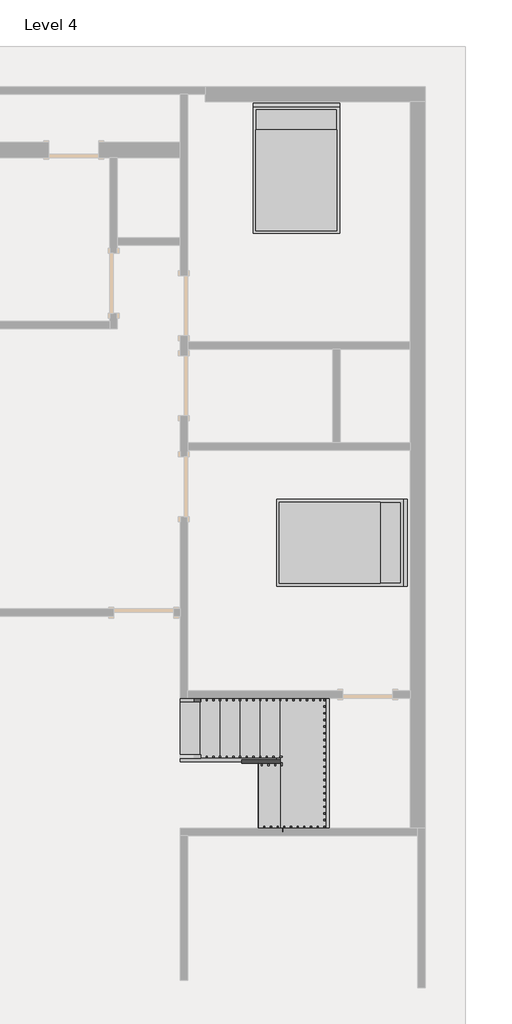
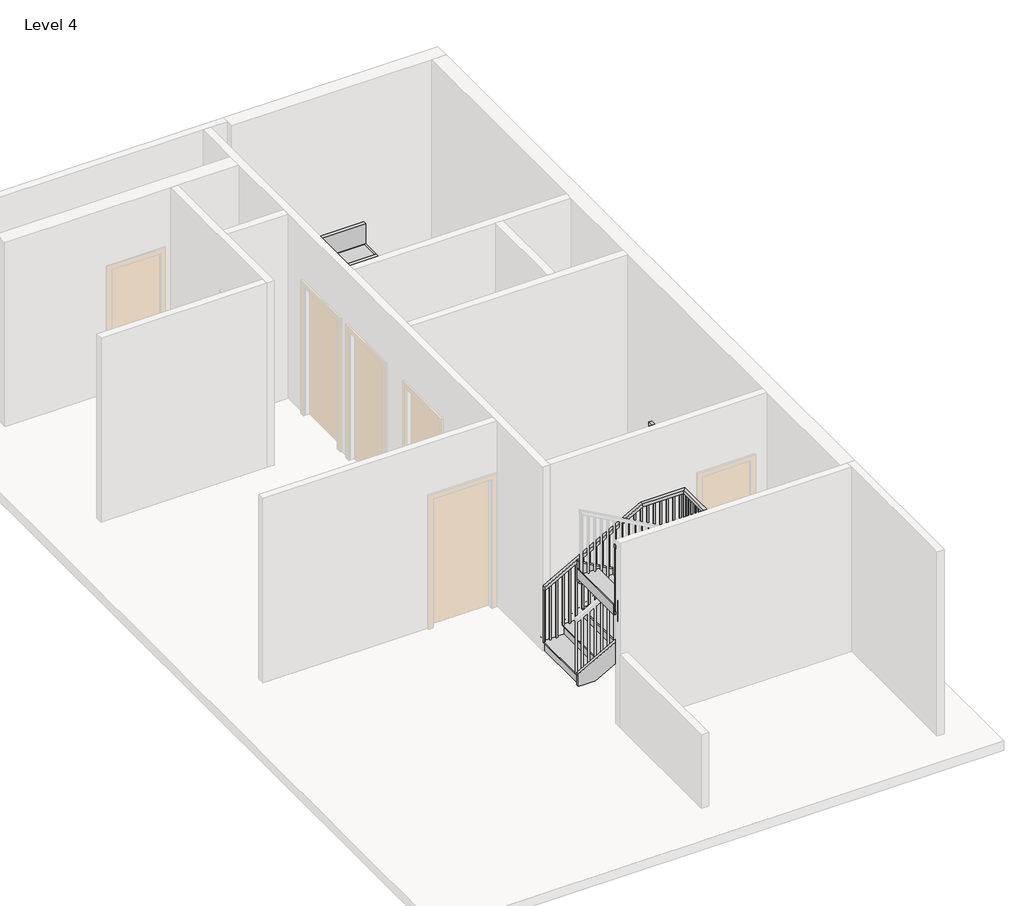
# One storey, part 2 of 2: 6 members, 2 furniture elements, 1 railing, 1 stair flight.
"""IFC4 building model written with IfcOpenShell, lengths in millimetres."""

from ifc_helpers import new_model, si_unit, frame, origin, place, context, project, spatial, polyline, outline, extrude, faceted_brep, transform, mapped, element, save
from components import bed_17739_bed_17739_15c61121, stair_flight_f370bc99

model = new_model("IFC4")

# Units and contexts
model_context = context("Model", 3, world=origin())
ifc_project = project(units=[si_unit("LENGTHUNIT", "METRE", prefix="MILLI")], contexts=[model_context])

# Site, building, storey
site = spatial("IfcSite", under=ifc_project)
building = spatial("IfcBuilding", under=site)
storey = spatial("IfcBuildingStorey", under=building, Name="Level 4", Elevation=6400.8)

# Furniture
placement = place(None, origin())
bed_17739_bed_17739_shape = bed_17739_bed_17739_15c61121(model_context)
element("IfcFurniture", 1, ObjectType="Bed_17739 : Bed_17739", at=placement, inside=storey, context=model_context, shape_type="MappedRepresentation", body=[
    mapped(bed_17739_bed_17739_shape, transform((592.6084916, 6126.1935985, 6400.8), x_axis=(1.0, 0.0, 0.0), y_axis=(0.0, 1.0, 0.0), z_axis=(0.0, 0.0, 1.0))),
])
element("IfcFurniture", 2, ObjectType="Bed_17739 : Bed_17739", at=placement, inside=storey, context=model_context, shape_type="MappedRepresentation", body=[
    mapped(bed_17739_bed_17739_shape, transform((1259.3584916, 455.6435985, 6400.8), x_axis=(0.0, -1.0, 0.0), y_axis=(1.0, 0.0, 0.0), z_axis=(0.0, 0.0, 1.0))),
])

# Members
element("IfcMember", 3, ObjectType="Stringer - 2\" Width", at=placement, inside=storey, context=model_context, shape_type="SweptSolid", body=[
    extrude(outline(polyline([(6608.3983948, -1179.0415084), (6400.8, -1179.0415084), (6400.8, -925.0970056), (7493.0, 1040.8629944), (7493.0, 413.241381), (6608.3983948, -1179.0415084)])), frame((0.0, -1912.9064015, 0.0), z_axis=(0.0, 1.0, 0.0), x_axis=(0.0, 0.0, 1.0)), (0.0, 0.0, 1.0), 50.8),
])
element("IfcMember", 4, ObjectType="Stringer - 2\" Width", at=placement, inside=storey, context=model_context, shape_type="SweptSolid", body=[
    extrude(outline(polyline([(1043.4584916, -1862.1064015), (1094.2584916, -1862.1064015), (1094.2584916, -3894.1064015), (1043.4584916, -3894.1064015), (1043.4584916, -1862.1064015)])), frame((0.0, 0.0, 7188.2), z_axis=(0.0, 0.0, 1.0), x_axis=(1.0, 0.0, 0.0)), (0.0, 0.0, 1.0), 304.8),
])
element("IfcMember", 5, ObjectType="Stringer - 2\" Width", at=placement, inside=storey, context=model_context, shape_type="SweptSolid", body=[
    extrude(outline(polyline([(7188.2, 1094.2584916), (7208.120617, 1094.2584916), (8471.0650614, -1179.0415084), (8122.3863873, -1179.0415084), (7188.2, 502.4939888), (7188.2, 1094.2584916)])), frame((0.0, -3944.9064015, 0.0), z_axis=(0.0, 1.0, 0.0), x_axis=(0.0, 0.0, 1.0)), (0.0, 0.0, 1.0), 50.8),
])
element("IfcMember", 6, ObjectType="Stringer - 2\" Width", at=placement, inside=storey, context=model_context, shape_type="SweptSolid", body=[
    extrude(outline(polyline([(6608.3983948, -1179.0415084), (6400.8, -1179.0415084), (6400.8, -925.0970056), (7078.1641651, 294.1584916), (7426.8428392, 294.1584916), (6608.3983948, -1179.0415084)])), frame((0.0, -2878.1064015, 0.0), z_axis=(0.0, 1.0, 0.0), x_axis=(0.0, 0.0, 1.0)), (0.0, 0.0, 1.0), 50.8),
])
element("IfcMember", 7, ObjectType="Stringer - 2\" Width", at=placement, inside=storey, context=model_context, shape_type="SweptSolid", body=[
    extrude(outline(polyline([(294.1584916, -2827.3064015), (344.9584916, -2827.3064015), (344.9584916, -2852.7064015), (294.1584916, -2852.7064015), (294.1584916, -2827.3064015)])), frame((0.0, 0.0, 7188.2), z_axis=(0.0, 0.0, 1.0), x_axis=(1.0, 0.0, 0.0)), (0.0, 0.0, 1.0), 304.8),
])
element("IfcMember", 8, ObjectType="Stringer - 2\" Width", at=placement, inside=storey, context=model_context, shape_type="SweptSolid", body=[
    extrude(outline(polyline([(7275.7197207, 344.9584916), (7624.3983948, 344.9584916), (8471.0650614, -1179.0415084), (8122.3863873, -1179.0415084), (7275.7197207, 344.9584916)])), frame((0.0, -2903.5064015, 0.0), z_axis=(0.0, 1.0, 0.0), x_axis=(0.0, 0.0, 1.0)), (0.0, 0.0, 1.0), 50.8),
])

# Railing
element("IfcRailing", 9, ObjectType="Handrail - Rectangular", at=placement, inside=storey, context=model_context, shape_type="SolidModel", body=[
    faceted_brep([(-1179.0415084, -1912.9064015, 7484.5333333), (-1179.0415084, -1912.9064015, 7426.420221), (-1179.0415084, -1963.7064015, 7426.420221), (-1179.0415084, -1963.7064015, 7484.5333333), (344.9584916, -1912.9064015, 8331.2), (358.1220938, -1912.9064015, 8280.4), (358.1220938, -1963.7064015, 8280.4), (344.9584916, -1963.7064015, 8331.2), (1043.4584916, -1912.9064015, 8331.2), (1043.4584916, -1912.9064015, 8280.4), (992.6584916, -1963.7064015, 8280.4), (992.6584916, -1963.7064015, 8331.2), (1043.4584916, -3894.1064015, 8331.2), (1043.4584916, -3894.1064015, 8280.4), (992.6584916, -3843.3064015, 8280.4), (992.6584916, -3843.3064015, 8331.2), (649.7584916, -3894.1064015, 8331.2), (636.5948894, -3894.1064015, 8280.4), (636.5948894, -3843.3064015, 8280.4), (649.7584916, -3843.3064015, 8331.2), (-1179.0415084, -3894.1064015, 9347.2), (-1179.0415084, -3843.3064015, 9347.2), (-1179.0415084, -3843.3064015, 9289.0868876), (-1179.0415084, -3894.1064015, 9289.0868876)], [[[0, 1, 2, 3]], [[1, 0, 4, 5]], [[2, 1, 5, 6]], [[3, 2, 6, 7]], [[0, 3, 7, 4]], [[5, 4, 8, 9]], [[6, 5, 9, 10]], [[7, 6, 10, 11]], [[4, 7, 11, 8]], [[9, 8, 12, 13]], [[10, 9, 13, 14]], [[11, 10, 14, 15]], [[8, 11, 15, 12]], [[13, 12, 16, 17]], [[14, 13, 17, 18]], [[15, 14, 18, 19]], [[12, 15, 19, 16]], [[20, 21, 22, 23]], [[17, 16, 20, 23]], [[18, 17, 23, 22]], [[19, 18, 22, 21]], [[16, 19, 21, 20]]]),
    extrude(outline(polyline([(9259.1007765, -1125.0665084), (8263.4666667, -1125.0665084), (8263.4666667, -1106.0165084), (9248.5174432, -1106.0165084), (9259.1007765, -1125.0665084)])), frame((0.0, -3878.2314015, 0.0), z_axis=(0.0, 1.0, 0.0), x_axis=(0.0, 0.0, 1.0)), (0.0, 0.0, 1.0), 19.05),
    extrude(outline(polyline([(9202.6563321, -1023.4665084), (8263.4666667, -1023.4665084), (8263.4666667, -1004.4165084), (9192.0729988, -1004.4165084), (9202.6563321, -1023.4665084)])), frame((0.0, -3878.2314015, 0.0), z_axis=(0.0, 1.0, 0.0), x_axis=(0.0, 0.0, 1.0)), (0.0, 0.0, 1.0), 19.05),
    extrude(outline(polyline([(9146.2118876, -921.8665084), (8263.4666667, -921.8665084), (8263.4666667, -902.8165084), (9135.6285543, -902.8165084), (9146.2118876, -921.8665084)])), frame((0.0, -3878.2314015, 0.0), z_axis=(0.0, 1.0, 0.0), x_axis=(0.0, 0.0, 1.0)), (0.0, 0.0, 1.0), 19.05),
    extrude(outline(polyline([(9089.7674432, -820.2665084), (8094.1333333, -820.2665084), (8094.1333333, -801.2165084), (9079.1841099, -801.2165084), (9089.7674432, -820.2665084)])), frame((0.0, -3878.2314015, 0.0), z_axis=(0.0, 1.0, 0.0), x_axis=(0.0, 0.0, 1.0)), (0.0, 0.0, 1.0), 19.05),
    extrude(outline(polyline([(9033.3229988, -718.6665084), (8094.1333333, -718.6665084), (8094.1333333, -699.6165084), (9022.7396654, -699.6165084), (9033.3229988, -718.6665084)])), frame((0.0, -3878.2314015, 0.0), z_axis=(0.0, 1.0, 0.0), x_axis=(0.0, 0.0, 1.0)), (0.0, 0.0, 1.0), 19.05),
    extrude(outline(polyline([(8976.8785543, -617.0665084), (8094.1333333, -617.0665084), (8094.1333333, -598.0165084), (8966.295221, -598.0165084), (8976.8785543, -617.0665084)])), frame((0.0, -3878.2314015, 0.0), z_axis=(0.0, 1.0, 0.0), x_axis=(0.0, 0.0, 1.0)), (0.0, 0.0, 1.0), 19.05),
    extrude(outline(polyline([(8920.4341099, -515.4665084), (7924.8, -515.4665084), (7924.8, -496.4165084), (8909.8507765, -496.4165084), (8920.4341099, -515.4665084)])), frame((0.0, -3878.2314015, 0.0), z_axis=(0.0, 1.0, 0.0), x_axis=(0.0, 0.0, 1.0)), (0.0, 0.0, 1.0), 19.05),
    extrude(outline(polyline([(8863.9896654, -413.8665084), (7924.8, -413.8665084), (7924.8, -394.8165084), (8853.4063321, -394.8165084), (8863.9896654, -413.8665084)])), frame((0.0, -3878.2314015, 0.0), z_axis=(0.0, 1.0, 0.0), x_axis=(0.0, 0.0, 1.0)), (0.0, 0.0, 1.0), 19.05),
    extrude(outline(polyline([(8807.545221, -312.2665084), (7924.8, -312.2665084), (7924.8, -293.2165084), (8796.9618876, -293.2165084), (8807.545221, -312.2665084)])), frame((0.0, -3878.2314015, 0.0), z_axis=(0.0, 1.0, 0.0), x_axis=(0.0, 0.0, 1.0)), (0.0, 0.0, 1.0), 19.05),
    extrude(outline(polyline([(8751.1007765, -210.6665084), (7755.4666667, -210.6665084), (7755.4666667, -191.6165084), (8740.5174432, -191.6165084), (8751.1007765, -210.6665084)])), frame((0.0, -3878.2314015, 0.0), z_axis=(0.0, 1.0, 0.0), x_axis=(0.0, 0.0, 1.0)), (0.0, 0.0, 1.0), 19.05),
    extrude(outline(polyline([(8694.6563321, -109.0665084), (7755.4666667, -109.0665084), (7755.4666667, -90.0165084), (8684.0729988, -90.0165084), (8694.6563321, -109.0665084)])), frame((0.0, -3878.2314015, 0.0), z_axis=(0.0, 1.0, 0.0), x_axis=(0.0, 0.0, 1.0)), (0.0, 0.0, 1.0), 19.05),
    extrude(outline(polyline([(8638.2118876, -7.4665084), (7755.4666667, -7.4665084), (7755.4666667, 11.5834916), (8627.6285543, 11.5834916), (8638.2118876, -7.4665084)])), frame((0.0, -3878.2314015, 0.0), z_axis=(0.0, 1.0, 0.0), x_axis=(0.0, 0.0, 1.0)), (0.0, 0.0, 1.0), 19.05),
    extrude(outline(polyline([(8581.7674432, 94.1334916), (7586.1333333, 94.1334916), (7586.1333333, 113.1834916), (8571.1841099, 113.1834916), (8581.7674432, 94.1334916)])), frame((0.0, -3878.2314015, 0.0), z_axis=(0.0, 1.0, 0.0), x_axis=(0.0, 0.0, 1.0)), (0.0, 0.0, 1.0), 19.05),
    extrude(outline(polyline([(8525.3229988, 195.7334916), (7586.1333333, 195.7334916), (7586.1333333, 214.7834916), (8514.7396654, 214.7834916), (8525.3229988, 195.7334916)])), frame((0.0, -3878.2314015, 0.0), z_axis=(0.0, 1.0, 0.0), x_axis=(0.0, 0.0, 1.0)), (0.0, 0.0, 1.0), 19.05),
    extrude(outline(polyline([(8468.8785543, 297.3334916), (7586.1333333, 297.3334916), (7586.1333333, 316.3834916), (8458.295221, 316.3834916), (8468.8785543, 297.3334916)])), frame((0.0, -3878.2314015, 0.0), z_axis=(0.0, 1.0, 0.0), x_axis=(0.0, 0.0, 1.0)), (0.0, 0.0, 1.0), 19.05),
    extrude(outline(polyline([(8412.4341099, 398.9334916), (7416.8, 398.9334916), (7416.8, 417.9834916), (8401.8507765, 417.9834916), (8412.4341099, 398.9334916)])), frame((0.0, -3878.2314015, 0.0), z_axis=(0.0, 1.0, 0.0), x_axis=(0.0, 0.0, 1.0)), (0.0, 0.0, 1.0), 19.05),
    extrude(outline(polyline([(8355.9896654, 500.5334916), (7416.8, 500.5334916), (7416.8, 519.5834916), (8345.4063321, 519.5834916), (8355.9896654, 500.5334916)])), frame((0.0, -3878.2314015, 0.0), z_axis=(0.0, 1.0, 0.0), x_axis=(0.0, 0.0, 1.0)), (0.0, 0.0, 1.0), 19.05),
    extrude(outline(polyline([(8299.545221, 602.1334916), (7416.8, 602.1334916), (7416.8, 621.1834916), (8288.9618876, 621.1834916), (8299.545221, 602.1334916)])), frame((0.0, -3878.2314015, 0.0), z_axis=(0.0, 1.0, 0.0), x_axis=(0.0, 0.0, 1.0)), (0.0, 0.0, 1.0), 19.05),
    extrude(outline(polyline([(722.7834916, -3878.2314015), (703.7334916, -3878.2314015), (703.7334916, -3859.1814015), (722.7834916, -3859.1814015), (722.7834916, -3878.2314015)])), frame((0.0, 0.0, 7416.8), z_axis=(0.0, 0.0, 1.0), x_axis=(1.0, 0.0, 0.0)), (0.0, 0.0, 1.0), 863.6),
    extrude(outline(polyline([(824.3834916, -3878.2314015), (805.3334916, -3878.2314015), (805.3334916, -3859.1814015), (824.3834916, -3859.1814015), (824.3834916, -3878.2314015)])), frame((0.0, 0.0, 7416.8), z_axis=(0.0, 0.0, 1.0), x_axis=(1.0, 0.0, 0.0)), (0.0, 0.0, 1.0), 863.6),
    extrude(outline(polyline([(925.9834916, -3878.2314015), (906.9334916, -3878.2314015), (906.9334916, -3859.1814015), (925.9834916, -3859.1814015), (925.9834916, -3878.2314015)])), frame((0.0, 0.0, 7416.8), z_axis=(0.0, 0.0, 1.0), x_axis=(1.0, 0.0, 0.0)), (0.0, 0.0, 1.0), 863.6),
    extrude(outline(polyline([(1027.5834916, -3757.5814015), (1027.5834916, -3776.6314015), (1008.5334916, -3776.6314015), (1008.5334916, -3757.5814015), (1027.5834916, -3757.5814015)])), frame((0.0, 0.0, 7416.8), z_axis=(0.0, 0.0, 1.0), x_axis=(1.0, 0.0, 0.0)), (0.0, 0.0, 1.0), 863.6),
    extrude(outline(polyline([(1027.5834916, -3655.9814015), (1027.5834916, -3675.0314015), (1008.5334916, -3675.0314015), (1008.5334916, -3655.9814015), (1027.5834916, -3655.9814015)])), frame((0.0, 0.0, 7416.8), z_axis=(0.0, 0.0, 1.0), x_axis=(1.0, 0.0, 0.0)), (0.0, 0.0, 1.0), 863.6),
    extrude(outline(polyline([(1027.5834916, -3554.3814015), (1027.5834916, -3573.4314015), (1008.5334916, -3573.4314015), (1008.5334916, -3554.3814015), (1027.5834916, -3554.3814015)])), frame((0.0, 0.0, 7416.8), z_axis=(0.0, 0.0, 1.0), x_axis=(1.0, 0.0, 0.0)), (0.0, 0.0, 1.0), 863.6),
    extrude(outline(polyline([(1027.5834916, -3452.7814015), (1027.5834916, -3471.8314015), (1008.5334916, -3471.8314015), (1008.5334916, -3452.7814015), (1027.5834916, -3452.7814015)])), frame((0.0, 0.0, 7416.8), z_axis=(0.0, 0.0, 1.0), x_axis=(1.0, 0.0, 0.0)), (0.0, 0.0, 1.0), 863.6),
    extrude(outline(polyline([(1027.5834916, -3351.1814015), (1027.5834916, -3370.2314015), (1008.5334916, -3370.2314015), (1008.5334916, -3351.1814015), (1027.5834916, -3351.1814015)])), frame((0.0, 0.0, 7416.8), z_axis=(0.0, 0.0, 1.0), x_axis=(1.0, 0.0, 0.0)), (0.0, 0.0, 1.0), 863.6),
    extrude(outline(polyline([(1027.5834916, -3249.5814015), (1027.5834916, -3268.6314015), (1008.5334916, -3268.6314015), (1008.5334916, -3249.5814015), (1027.5834916, -3249.5814015)])), frame((0.0, 0.0, 7416.8), z_axis=(0.0, 0.0, 1.0), x_axis=(1.0, 0.0, 0.0)), (0.0, 0.0, 1.0), 863.6),
    extrude(outline(polyline([(1027.5834916, -3147.9814015), (1027.5834916, -3167.0314015), (1008.5334916, -3167.0314015), (1008.5334916, -3147.9814015), (1027.5834916, -3147.9814015)])), frame((0.0, 0.0, 7416.8), z_axis=(0.0, 0.0, 1.0), x_axis=(1.0, 0.0, 0.0)), (0.0, 0.0, 1.0), 863.6),
    extrude(outline(polyline([(1027.5834916, -3046.3814015), (1027.5834916, -3065.4314015), (1008.5334916, -3065.4314015), (1008.5334916, -3046.3814015), (1027.5834916, -3046.3814015)])), frame((0.0, 0.0, 7416.8), z_axis=(0.0, 0.0, 1.0), x_axis=(1.0, 0.0, 0.0)), (0.0, 0.0, 1.0), 863.6),
    extrude(outline(polyline([(1027.5834916, -2944.7814015), (1027.5834916, -2963.8314015), (1008.5334916, -2963.8314015), (1008.5334916, -2944.7814015), (1027.5834916, -2944.7814015)])), frame((0.0, 0.0, 7416.8), z_axis=(0.0, 0.0, 1.0), x_axis=(1.0, 0.0, 0.0)), (0.0, 0.0, 1.0), 863.6),
    extrude(outline(polyline([(1027.5834916, -2843.1814015), (1027.5834916, -2862.2314015), (1008.5334916, -2862.2314015), (1008.5334916, -2843.1814015), (1027.5834916, -2843.1814015)])), frame((0.0, 0.0, 7416.8), z_axis=(0.0, 0.0, 1.0), x_axis=(1.0, 0.0, 0.0)), (0.0, 0.0, 1.0), 863.6),
    extrude(outline(polyline([(1027.5834916, -2741.5814015), (1027.5834916, -2760.6314015), (1008.5334916, -2760.6314015), (1008.5334916, -2741.5814015), (1027.5834916, -2741.5814015)])), frame((0.0, 0.0, 7416.8), z_axis=(0.0, 0.0, 1.0), x_axis=(1.0, 0.0, 0.0)), (0.0, 0.0, 1.0), 863.6),
    extrude(outline(polyline([(1027.5834916, -2639.9814015), (1027.5834916, -2659.0314015), (1008.5334916, -2659.0314015), (1008.5334916, -2639.9814015), (1027.5834916, -2639.9814015)])), frame((0.0, 0.0, 7416.8), z_axis=(0.0, 0.0, 1.0), x_axis=(1.0, 0.0, 0.0)), (0.0, 0.0, 1.0), 863.6),
    extrude(outline(polyline([(1027.5834916, -2538.3814015), (1027.5834916, -2557.4314015), (1008.5334916, -2557.4314015), (1008.5334916, -2538.3814015), (1027.5834916, -2538.3814015)])), frame((0.0, 0.0, 7416.8), z_axis=(0.0, 0.0, 1.0), x_axis=(1.0, 0.0, 0.0)), (0.0, 0.0, 1.0), 863.6),
    extrude(outline(polyline([(1027.5834916, -2436.7814015), (1027.5834916, -2455.8314015), (1008.5334916, -2455.8314015), (1008.5334916, -2436.7814015), (1027.5834916, -2436.7814015)])), frame((0.0, 0.0, 7416.8), z_axis=(0.0, 0.0, 1.0), x_axis=(1.0, 0.0, 0.0)), (0.0, 0.0, 1.0), 863.6),
    extrude(outline(polyline([(1027.5834916, -2335.1814015), (1027.5834916, -2354.2314015), (1008.5334916, -2354.2314015), (1008.5334916, -2335.1814015), (1027.5834916, -2335.1814015)])), frame((0.0, 0.0, 7416.8), z_axis=(0.0, 0.0, 1.0), x_axis=(1.0, 0.0, 0.0)), (0.0, 0.0, 1.0), 863.6),
    extrude(outline(polyline([(1027.5834916, -2233.5814015), (1027.5834916, -2252.6314015), (1008.5334916, -2252.6314015), (1008.5334916, -2233.5814015), (1027.5834916, -2233.5814015)])), frame((0.0, 0.0, 7416.8), z_axis=(0.0, 0.0, 1.0), x_axis=(1.0, 0.0, 0.0)), (0.0, 0.0, 1.0), 863.6),
    extrude(outline(polyline([(1027.5834916, -2131.9814015), (1027.5834916, -2151.0314015), (1008.5334916, -2151.0314015), (1008.5334916, -2131.9814015), (1027.5834916, -2131.9814015)])), frame((0.0, 0.0, 7416.8), z_axis=(0.0, 0.0, 1.0), x_axis=(1.0, 0.0, 0.0)), (0.0, 0.0, 1.0), 863.6),
    extrude(outline(polyline([(1027.5834916, -2030.3814015), (1027.5834916, -2049.4314015), (1008.5334916, -2049.4314015), (1008.5334916, -2030.3814015), (1027.5834916, -2030.3814015)])), frame((0.0, 0.0, 7416.8), z_axis=(0.0, 0.0, 1.0), x_axis=(1.0, 0.0, 0.0)), (0.0, 0.0, 1.0), 863.6),
    extrude(outline(polyline([(945.0334916, -1928.7814015), (964.0834916, -1928.7814015), (964.0834916, -1947.8314015), (945.0334916, -1947.8314015), (945.0334916, -1928.7814015)])), frame((0.0, 0.0, 7416.8), z_axis=(0.0, 0.0, 1.0), x_axis=(1.0, 0.0, 0.0)), (0.0, 0.0, 1.0), 863.6),
    extrude(outline(polyline([(843.4334916, -1928.7814015), (862.4834916, -1928.7814015), (862.4834916, -1947.8314015), (843.4334916, -1947.8314015), (843.4334916, -1928.7814015)])), frame((0.0, 0.0, 7416.8), z_axis=(0.0, 0.0, 1.0), x_axis=(1.0, 0.0, 0.0)), (0.0, 0.0, 1.0), 863.6),
    extrude(outline(polyline([(741.8334916, -1928.7814015), (760.8834916, -1928.7814015), (760.8834916, -1947.8314015), (741.8334916, -1947.8314015), (741.8334916, -1928.7814015)])), frame((0.0, 0.0, 7416.8), z_axis=(0.0, 0.0, 1.0), x_axis=(1.0, 0.0, 0.0)), (0.0, 0.0, 1.0), 863.6),
    extrude(outline(polyline([(640.2334916, -1928.7814015), (659.2834916, -1928.7814015), (659.2834916, -1947.8314015), (640.2334916, -1947.8314015), (640.2334916, -1928.7814015)])), frame((0.0, 0.0, 7416.8), z_axis=(0.0, 0.0, 1.0), x_axis=(1.0, 0.0, 0.0)), (0.0, 0.0, 1.0), 863.6),
    extrude(outline(polyline([(538.6334916, -1928.7814015), (557.6834916, -1928.7814015), (557.6834916, -1947.8314015), (538.6334916, -1947.8314015), (538.6334916, -1928.7814015)])), frame((0.0, 0.0, 7416.8), z_axis=(0.0, 0.0, 1.0), x_axis=(1.0, 0.0, 0.0)), (0.0, 0.0, 1.0), 863.6),
    extrude(outline(polyline([(437.0334916, -1928.7814015), (456.0834916, -1928.7814015), (456.0834916, -1947.8314015), (437.0334916, -1947.8314015), (437.0334916, -1928.7814015)])), frame((0.0, 0.0, 7416.8), z_axis=(0.0, 0.0, 1.0), x_axis=(1.0, 0.0, 0.0)), (0.0, 0.0, 1.0), 863.6),
    extrude(outline(polyline([(8267.795221, 335.4334916), (7416.8, 335.4334916), (7416.8, 354.4834916), (8278.3785543, 354.4834916), (8267.795221, 335.4334916)])), frame((0.0, -1947.8314015, 0.0), z_axis=(0.0, 1.0, 0.0), x_axis=(0.0, 0.0, 1.0)), (0.0, 0.0, 1.0), 19.05),
    extrude(outline(polyline([(8211.3507765, 233.8334916), (7247.4666667, 233.8334916), (7247.4666667, 252.8834916), (8221.9341099, 252.8834916), (8211.3507765, 233.8334916)])), frame((0.0, -1947.8314015, 0.0), z_axis=(0.0, 1.0, 0.0), x_axis=(0.0, 0.0, 1.0)), (0.0, 0.0, 1.0), 19.05),
    extrude(outline(polyline([(8154.9063321, 132.2334916), (7247.4666667, 132.2334916), (7247.4666667, 151.2834916), (8165.4896654, 151.2834916), (8154.9063321, 132.2334916)])), frame((0.0, -1947.8314015, 0.0), z_axis=(0.0, 1.0, 0.0), x_axis=(0.0, 0.0, 1.0)), (0.0, 0.0, 1.0), 19.05),
    extrude(outline(polyline([(8098.4618876, 30.6334916), (7247.4666667, 30.6334916), (7247.4666667, 49.6834916), (8109.045221, 49.6834916), (8098.4618876, 30.6334916)])), frame((0.0, -1947.8314015, 0.0), z_axis=(0.0, 1.0, 0.0), x_axis=(0.0, 0.0, 1.0)), (0.0, 0.0, 1.0), 19.05),
    extrude(outline(polyline([(8042.0174432, -70.9665084), (7078.1333333, -70.9665084), (7078.1333333, -51.9165084), (8052.6007765, -51.9165084), (8042.0174432, -70.9665084)])), frame((0.0, -1947.8314015, 0.0), z_axis=(0.0, 1.0, 0.0), x_axis=(0.0, 0.0, 1.0)), (0.0, 0.0, 1.0), 19.05),
    extrude(outline(polyline([(7985.5729988, -172.5665084), (7078.1333333, -172.5665084), (7078.1333333, -153.5165084), (7996.1563321, -153.5165084), (7985.5729988, -172.5665084)])), frame((0.0, -1947.8314015, 0.0), z_axis=(0.0, 1.0, 0.0), x_axis=(0.0, 0.0, 1.0)), (0.0, 0.0, 1.0), 19.05),
    extrude(outline(polyline([(7929.1285543, -274.1665084), (7078.1333333, -274.1665084), (7078.1333333, -255.1165084), (7939.7118876, -255.1165084), (7929.1285543, -274.1665084)])), frame((0.0, -1947.8314015, 0.0), z_axis=(0.0, 1.0, 0.0), x_axis=(0.0, 0.0, 1.0)), (0.0, 0.0, 1.0), 19.05),
    extrude(outline(polyline([(7872.6841099, -375.7665084), (6908.8, -375.7665084), (6908.8, -356.7165084), (7883.2674432, -356.7165084), (7872.6841099, -375.7665084)])), frame((0.0, -1947.8314015, 0.0), z_axis=(0.0, 1.0, 0.0), x_axis=(0.0, 0.0, 1.0)), (0.0, 0.0, 1.0), 19.05),
    extrude(outline(polyline([(7816.2396654, -477.3665084), (6908.8, -477.3665084), (6908.8, -458.3165084), (7826.8229988, -458.3165084), (7816.2396654, -477.3665084)])), frame((0.0, -1947.8314015, 0.0), z_axis=(0.0, 1.0, 0.0), x_axis=(0.0, 0.0, 1.0)), (0.0, 0.0, 1.0), 19.05),
    extrude(outline(polyline([(7759.795221, -578.9665084), (6908.8, -578.9665084), (6908.8, -559.9165084), (7770.3785543, -559.9165084), (7759.795221, -578.9665084)])), frame((0.0, -1947.8314015, 0.0), z_axis=(0.0, 1.0, 0.0), x_axis=(0.0, 0.0, 1.0)), (0.0, 0.0, 1.0), 19.05),
    extrude(outline(polyline([(7703.3507765, -680.5665084), (6739.4666667, -680.5665084), (6739.4666667, -661.5165084), (7713.9341099, -661.5165084), (7703.3507765, -680.5665084)])), frame((0.0, -1947.8314015, 0.0), z_axis=(0.0, 1.0, 0.0), x_axis=(0.0, 0.0, 1.0)), (0.0, 0.0, 1.0), 19.05),
    extrude(outline(polyline([(7646.9063321, -782.1665084), (6739.4666667, -782.1665084), (6739.4666667, -763.1165084), (7657.4896654, -763.1165084), (7646.9063321, -782.1665084)])), frame((0.0, -1947.8314015, 0.0), z_axis=(0.0, 1.0, 0.0), x_axis=(0.0, 0.0, 1.0)), (0.0, 0.0, 1.0), 19.05),
    extrude(outline(polyline([(7590.4618876, -883.7665084), (6739.4666667, -883.7665084), (6739.4666667, -864.7165084), (7601.045221, -864.7165084), (7590.4618876, -883.7665084)])), frame((0.0, -1947.8314015, 0.0), z_axis=(0.0, 1.0, 0.0), x_axis=(0.0, 0.0, 1.0)), (0.0, 0.0, 1.0), 19.05),
    extrude(outline(polyline([(7534.0174432, -985.3665084), (6570.1333333, -985.3665084), (6570.1333333, -966.3165084), (7544.6007765, -966.3165084), (7534.0174432, -985.3665084)])), frame((0.0, -1947.8314015, 0.0), z_axis=(0.0, 1.0, 0.0), x_axis=(0.0, 0.0, 1.0)), (0.0, 0.0, 1.0), 19.05),
    extrude(outline(polyline([(7477.5729988, -1086.9665084), (6570.1333333, -1086.9665084), (6570.1333333, -1067.9165084), (7488.1563321, -1067.9165084), (7477.5729988, -1086.9665084)])), frame((0.0, -1947.8314015, 0.0), z_axis=(0.0, 1.0, 0.0), x_axis=(0.0, 0.0, 1.0)), (0.0, 0.0, 1.0), 19.05),
    extrude(outline(polyline([(1027.5834916, -3859.1814015), (1027.5834916, -3878.2314015), (1008.5334916, -3878.2314015), (1008.5334916, -3859.1814015), (1027.5834916, -3859.1814015)])), frame((0.0, 0.0, 7416.8), z_axis=(0.0, 0.0, 1.0), x_axis=(1.0, 0.0, 0.0)), (0.0, 0.0, 1.0), 863.6),
    extrude(outline(polyline([(1008.5334916, -1928.7814015), (1027.5834916, -1928.7814015), (1027.5834916, -1947.8314015), (1008.5334916, -1947.8314015), (1008.5334916, -1928.7814015)])), frame((0.0, 0.0, 7416.8), z_axis=(0.0, 0.0, 1.0), x_axis=(1.0, 0.0, 0.0)), (0.0, 0.0, 1.0), 863.6),
    extrude(outline(polyline([(9289.0868876, -1179.0415084), (8263.4666667, -1179.0415084), (8263.4666667, -1159.9915084), (9278.5035543, -1159.9915084), (9289.0868876, -1179.0415084)])), frame((0.0, -3878.2314015, 0.0), z_axis=(0.0, 1.0, 0.0), x_axis=(0.0, 0.0, 1.0)), (0.0, 0.0, 1.0), 19.05),
    extrude(outline(polyline([(7426.420221, -1179.0415084), (6570.1333333, -1179.0415084), (6570.1333333, -1159.9915084), (7437.0035543, -1159.9915084), (7426.420221, -1179.0415084)])), frame((0.0, -1947.8314015, 0.0), z_axis=(0.0, 1.0, 0.0), x_axis=(0.0, 0.0, 1.0)), (0.0, 0.0, 1.0), 19.05),
])

# Stair flight
stair_flight_shape = stair_flight_f370bc99(model_context)
element("IfcStairFlight", 10, ObjectType="2\" Tread 1\" Nosing 1/4\" Riser", at=placement, inside=storey, context=model_context, shape_type="MappedRepresentation", body=[
    mapped(stair_flight_shape, transform((0.0, 0.0, 0.0), x_axis=(1.0, 0.0, 0.0), y_axis=(0.0, 1.0, 0.0), z_axis=(0.0, 0.0, 1.0))),
])

save(model, "model.ifc")

# Revit data of these elements
# Type "Bed_17739 : Bed_17739"
#   Default Elevation = 0
# Type "Handrail - Rectangular"
#   Assembly Code = "C2010400"
#   built-in parameter 1008612 = 0.0416667 (stored number, unit not read)
#   built-in parameter 1008611 = 0.0416667 (stored number, unit not read)
#   built-in parameter 1008609 = 0.333333 (stored number, unit not read)
#   built-in parameter 1008604 = 0.166667 (stored number, unit not read)
#   built-in parameter 1008603 = 0.166667 (stored number, unit not read)
#   Railing Height = 3' - 0"
#   built-in parameter 1008630 = 2
#   built-in parameter 1008610 = 2
#   built-in parameter 1008618 = Baluster - Square : 3/4"
# Elements 1, 2 (IfcFurniture, "Bed_17739 : Bed_17739")
#   Phase Created = New Construction
#   Materials on its faces: "legs", "sheets", "bed frame", "Blanket"
# Elements 3, 4, 5, 6, 7, 8 (IfcMember, "Stringer - 2\" Width")
#   Phase Created = New Construction
# Element 9 (IfcRailing, "Handrail - Rectangular")
#   Phase Created = New Construction
# Element 10 (IfcStairFlight, "2\" Tread 1\" Nosing 1/4\" Riser")
#   Phase Created = New Construction
# Materials
#   "legs": colour RGB 90 73 37, transparency 0, Cost = 0
#   "sheets": colour RGB 200 195 176, transparency 0, Cost = 0
#   "bed frame": colour RGB 90 73 37, transparency 0, Cost = 0
#   "Blanket": class "System", colour RGB 59 0 1, transparency 0, Cost = 0
